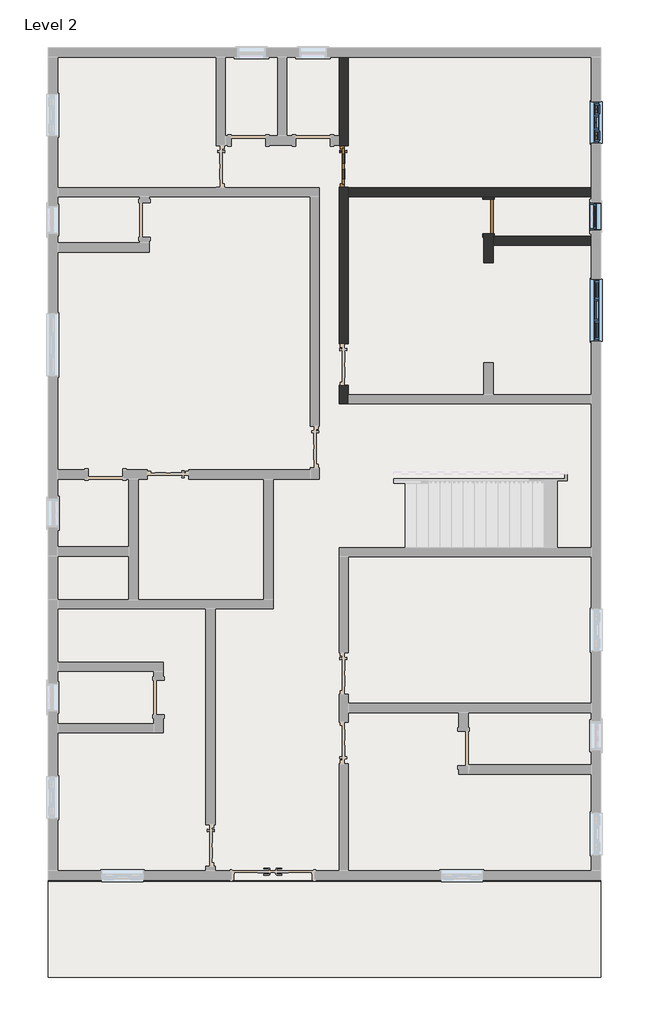
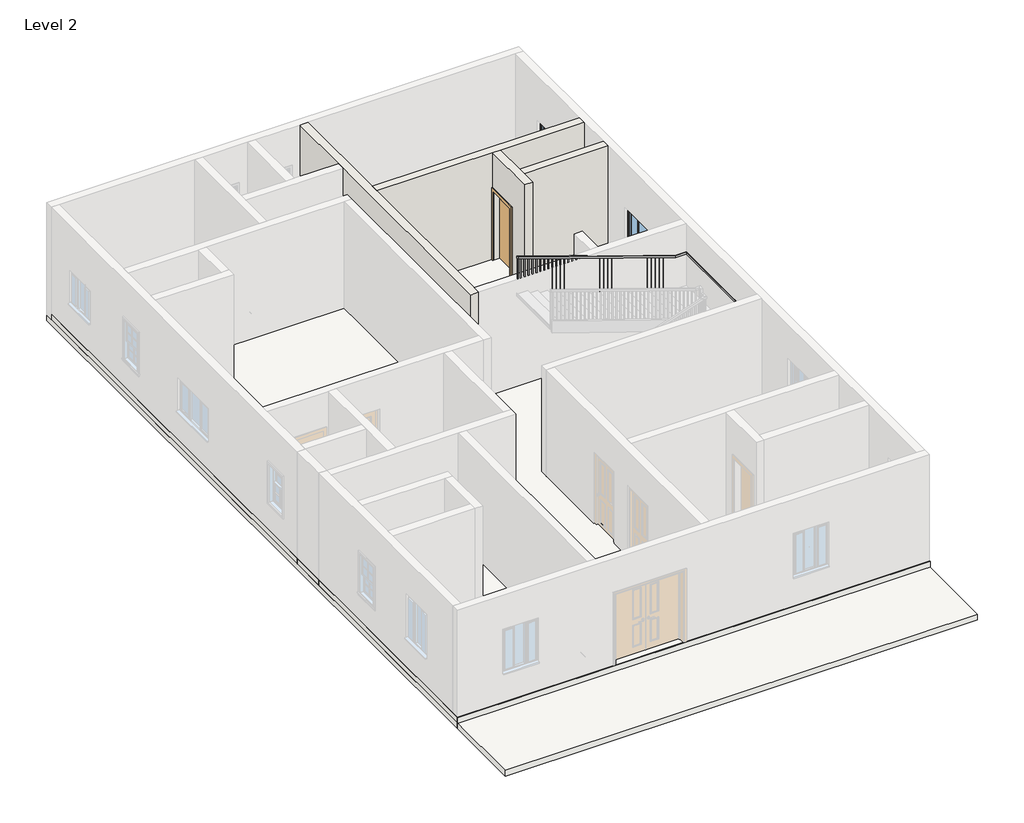
# One storey, part 2 of 3: 4 walls, 3 windows, 2 doors, 2 roofs, 2 slabs, 1 railing.
# Revit data of these elements (continued)
# Type "Windows_Tpl_w-Glazing_Cross-Bars : 910x910mm" (continued)
#   Wrap Layers (Int) from Ext = 0' - 6.98819"
#   Window Board Projection = 0' - 0.98425"
#   Window Board Extension = 0' - 0.98425"
#   Visual Light Transmittance = 0.9
#   Solar Heat Gain Coefficient = 0.78
#   Rough Width = 2' - 11.82677"
#   Rough Height = 2' - 11.82677"
#   Height = 2' - 11.82677"
#   Width = 2' - 11.82677"
#   Heat Transfer Coefficient (U) = 0.6496 BTU/(h·ft²·°F)
#   Glazing Thickness = 0' - 0.94488"
#   Glazing Bar Thickness = 0' - 0.7874"
#   FrameOffset - External = 0' - 1.9685"
#   Frame Depth = 0' - 2.55906"
#   Default Head Height = 6' - 11.07087"
#   Cill Depth = 0' - 3.44488"
#   Cavity Closer Width = 0' - 1.9685"
#   Cavity Closer Offset from Ext = 0' - 4.03543"
#   Cavity Closer Depth = 0' - 3.34646"
#   Vis - Glazing Bars = yes
#   Vis - Cavity Closers = yes
#   Define Thermal Properties by = 1
#   Material Trim = Window Frame
#   Material Glazing Bars = Window Frame
#   Material Glass = Glass
#   Material Frame = Window Frame
#   Wall Closure = (empty or 0)
# Element 1 (IfcDoor, "Doors_ExtSgl_2 : 2'x7\"")
#   Phase Created = New Construction
#   Materials on its faces: "Door - Panel", "Door - Handle", "Door - Frame/Mullion", "Door - Glazing"
# Element 2 (IfcDoor, "Single-Flush : 30\" x 80\"")
#   Phase Created = New Construction
#   Materials on its faces: "Door - Frame", "Door - Panel"
# Element 3 (IfcRailing, "Handrail - Rectangular")
#   Phase Created = New Construction
# Element 4 (IfcRoof, "Generic - 12\"")
#   built-in parameter 1001705 = 10.5 (stored number, unit not read)
#   built-in parameter 1001710 = 33615
#   Phase Created = New Construction
#   Materials on its faces: "Default Roof"
# Element 5 (IfcRoof, "Generic - 12\"")
#   built-in parameter 1001705 = 10.5 (stored number, unit not read)
#   built-in parameter 1001710 = 33615
#   Phase Created = New Construction
#   Materials on its faces: "Default Roof", "Door - Panel"
# Element 6 (IfcSlab, "Generic - 12\"")
#   Height Offset From Level = 0' - 0"
#   Phase Created = New Construction
#   Materials on its faces: "Default Floor"
# Element 7 (IfcSlab, "Generic - 12\"")
#   Height Offset From Level = 0' - 0"
#   Phase Created = New Construction
#   Materials on its faces: "Default Floor", "Window Frame"
# Elements 8, 9, 10, 11 (IfcWall, "Generic - 4.5\" p")
#   Top Offset = 0' - 0"
#   Base Offset = 0' - 0"
#   Unconnected Height = 10' - 0"
#   wall height = 10' - 0"
#   Phase Created = New Construction
#   Base Constraint = Level 2
#   Materials on its faces: "Default Wall"
# Element 12 (IfcWindow, "Window-Double-Hung : 24\" x 42\"")
#   Mark = "13"
#   Window Inset = 0' - 0"
#   Interior Wall Closure = 0' - 1 1/2"
#   Frame Extension = 0' - 1 1/4"
#   Exterior Wall Closure = 0' - 0 1/2"
#   Interior Trim Visibility = yes
#   Indicator Visibility = yes
#   Exterior Trim Visibility = yes
#   Phase Created = New Construction
#   Materials on its faces: "Wood - Stained", "Glass", "Clad - White"
# Element 13 (IfcWindow, "Windows_Tpl_Plain : 1360x910mm")
#   Mark = "6"
#   Phase Created = New Construction
#   Materials on its faces: "Window Frame", "Glass"
# Element 14 (IfcWindow, "Windows_Tpl_w-Glazing_Cross-Bars : 910x910mm")
#   Mark = "9"
#   Phase Created = New Construction
#   Materials on its faces: "Window Frame", "Glass"
# Materials
#   "Door - Glazing": colour RGB 0 0 255, transparency 0.75
#   "Door - Panel": class "Wood", colour RGB 210 159 95, transparency 0, Cost = 0
#   "Door - Frame/Mullion": class "Wood", colour RGB 212 179 113, transparency 0
#   "Door - Handle": colour RGB 246 240 166, transparency 0
#   "Door - Frame": colour RGB 118 70 51, transparency 0, Cost = 0
#   "Wood - Stained": class "Wood", colour RGB 224 178 126, transparency 0, Cost = 0
#   "Clad - White": class "Wood", colour RGB 242 242 238, transparency 0, Cost = 0
#   "Glass": class "Glass", colour RGB 0 128 192, transparency 0.75, Description = "Soda Lime Glass", Cost = 0
#   "Window Frame": colour RGB 249 249 249, transparency 0
#   "Default Roof": colour RGB 88 101 114, transparency 0, Cost = 0
#   "Default Floor": colour RGB 128 128 128, transparency 0, Cost = 0
#   "Default Wall": colour RGB 128 128 128, transparency 0, Cost = 0
